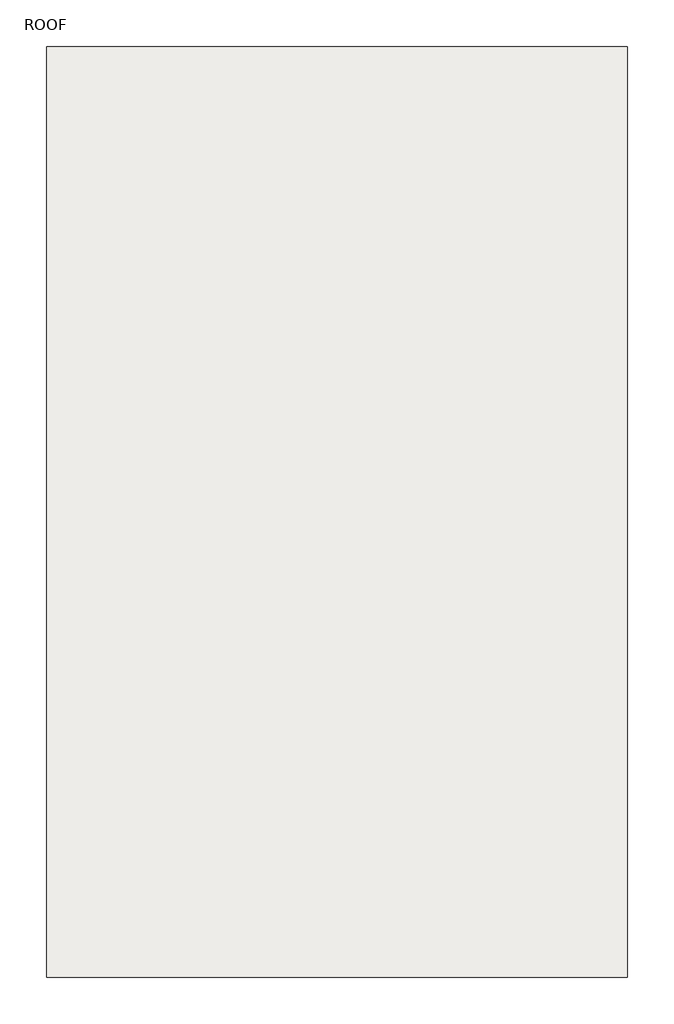
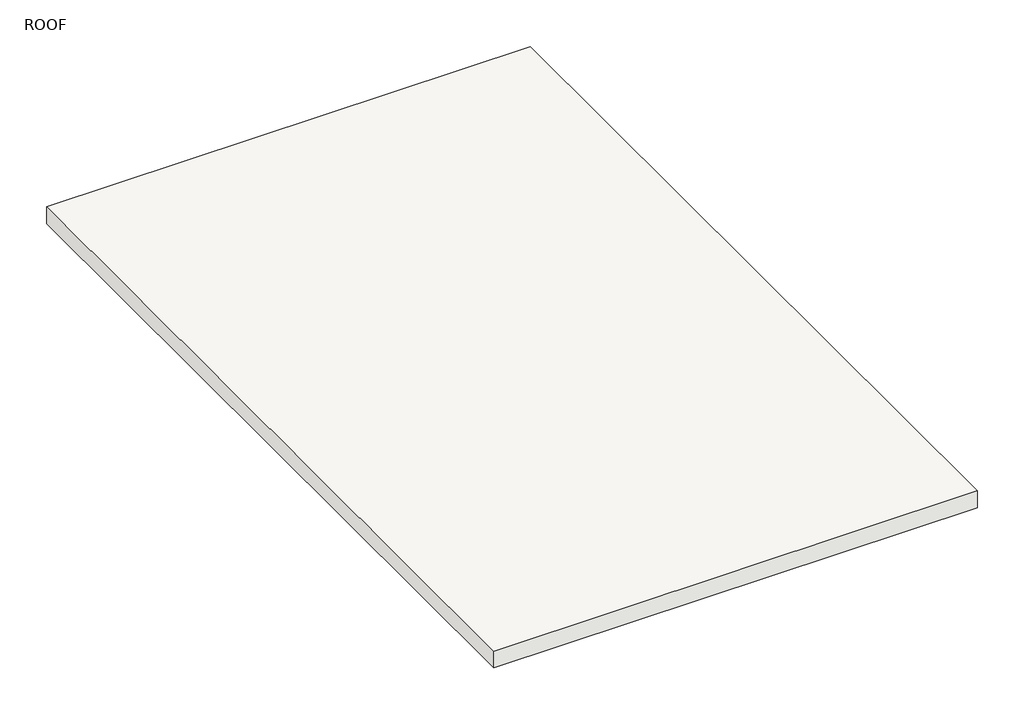
# One storey: 1 slab.
"""IFC4 building model written with IfcOpenShell, lengths in millimetres."""

from ifc_helpers import new_model, si_unit, frame, origin, place, context, project, spatial, polyline, outline, extrude, element, save

model = new_model("IFC4")

# Units and contexts
model_context = context("Model", 3, world=origin())
ifc_project = project(units=[si_unit("LENGTHUNIT", "METRE", prefix="MILLI")], contexts=[model_context])

# Site, building, storey
site = spatial("IfcSite", under=ifc_project)
building = spatial("IfcBuilding", under=site)
storey = spatial("IfcBuildingStorey", under=building, Name="ROOF", Elevation=9601.2)

# Slab
placement = place(None, origin())
element("IfcSlab", 1, ObjectType="6\"", at=placement, inside=storey, context=model_context, shape_type="SweptSolid", body=[
    extrude(outline(polyline([(-13501.0209734, 4430.0170657), (-9386.2209734, 4430.0170657), (-9386.2209734, -2161.2829343), (-13501.0209734, -2161.2829343), (-13501.0209734, 4430.0170657)])), frame((0.0, 0.0, 9448.8), z_axis=(0.0, 0.0, 1.0), x_axis=(1.0, 0.0, 0.0)), (0.0, 0.0, 1.0), 152.4),
])

save(model, "model.ifc")

# Revit data of these elements
# Type "6\""
#   Assembly Code = "B1010"
#   Function = 0
#   Layers, outside or top first: 0' - 6" no material (function 1)
# Element 1 (IfcSlab, "6\"")
#   built-in parameter 1001955 = 3.14159 (stored number, unit not read)
#   Height Offset From Level = 0' - 0"
#   Phase Created = New Construction
#   Materials on its faces: "Default Floor", "EIFS, Exterior Insulation"
# Materials
#   "Default Floor": colour RGB 128 128 128, transparency 0, Cost = 0
#   "EIFS, Exterior Insulation": class "Generic", colour RGB 127 127 127, transparency 0, Description = "EIFS - Exterior Insulation", Cost = 0
